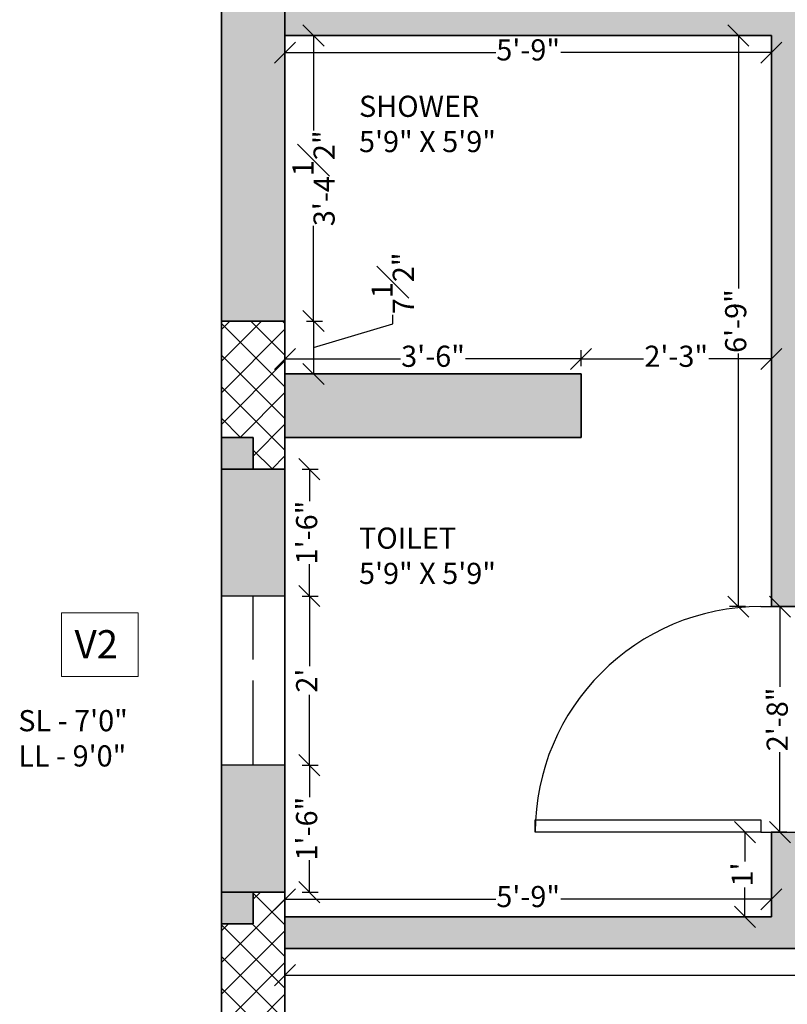
# Model space of a CAD drawing. Units: inches. Extents: x 1365 to 2091, y 1589 to 2091.
# Tile 2 of 8: x 1365 to 1474, y 1792 to 1932. Entities that reach past the tile are written whole.
import ezdxf

# ---------------------------------------------------------------- set-up
doc = ezdxf.new("R2010")
doc.units = ezdxf.units.IN
doc.linetypes.add('ACAD_ISO02W100', pattern=[15, 12, -3])
for name, color, linetype, lineweight in [('A-ANNO-DIMS', 2, 'Continuous', 18), ('A-ANNO-SYMB', 12, 'Continuous', 18), ('A-AREA-IDEN', 7, 'Continuous', 18), ('A-COLS', 7, 'Continuous', 35), ('A-COLS-MARK-PATT', 114, 'Continuous', 13), ('A-COLS-PATT', 1, 'Continuous', 13), ('A-DOOR', 4, 'Continuous', 25), ('A-GLAZ', 150, 'Continuous', 30), ('A-GLAZ-HIDN', 150, 'ACAD_ISO02W100', 30), ('A-WALL', 7, 'Continuous', 35), ('A-WALL-PATT', 253, 'Continuous', 13)]:
    doc.layers.add(name, color=color, linetype=linetype, lineweight=lineweight)
doc.styles.get("Standard").update_dxf_attribs({"font": 'arial.ttf'})
doc.dimstyles.new('ISO-25', dxfattribs={"dimtxt": 3, "dimasz": 3, "dimexe": 1.25, "dimexo": 0.625, "dimtad": 0, "dimlunit": 4, "dimtxsty": 'Standard', "dimblk": 'OBLIQUE', "dimcen": 2.5, "dimclrd": 254, "dimclre": 254, "dimclrt": 1, "dimadec": 0, "dimazin": 0, "dimtfac": 1, "dimtmove": 0, "dimatfit": 3, "dimfxl": 1, "dimfxlon": 1, "dimfrac": 1, "dimarcsym": 0})

# ---------------------------------------------------------------- blocks, each defined once
blk = doc.blocks.new('*U4')
for p, q in [((0, 0), (0, -6)), ((32, 0), (32, -6))]:
    blk.add_line(p, q)
blk.add_lwpolyline([(0, 0), (0, 32), (1.75, 32), (1.75, 0)], close=True)
blk.add_arc((0, 0), 32, 0, 90)
blk = doc.blocks.new('_Oblique')
at = {"color": 0, "linetype": 'ByBlock', "lineweight": -2}
blk.add_line((-0.5, -0.5), (0.5, 0.5), dxfattribs=at)
blk = doc.blocks.new('*D23')
at = {"layer": 'A-ANNO-DIMS', "color": 0, "lineweight": -2, "transparency": 16777216}
for p, q in [((1402.75, 1927.94), (1402.75, 1925.69)), ((1471.75, 1927.94), (1471.75, 1925.69)), ((1402.75, 1926.94), (1432.64, 1926.94)), ((1471.75, 1926.94), (1441.87, 1926.94))]:
    blk.add_line(p, q, dxfattribs=at)
at = {"layer": 'Defpoints', "color": 0, "transparency": 16777216}
for p in [(1402.75, 1929.36), (1471.75, 1929.36), (1471.75, 1926.94)]:
    blk.add_point(p, dxfattribs=at)
at = {"layer": 'A-ANNO-DIMS', "color": 0, "lineweight": -2, "transparency": 16777216, "xscale": 3, "yscale": 3, "zscale": 3, "rotation": 180}
blk.add_blockref('_Oblique', (1402.75, 1926.94), dxfattribs=at)
at = {"layer": 'A-ANNO-DIMS', "color": 0, "lineweight": -2, "transparency": 16777216, "xscale": 3, "yscale": 3, "zscale": 3}
blk.add_blockref('_Oblique', (1471.75, 1926.94), dxfattribs=at)
at = {"layer": 'A-ANNO-DIMS', "color": 0, "transparency": 16777216, "insert": (1437.25, 1926.94), "char_height": 3, "attachment_point": 5}
blk.add_mtext('5\'-9"', dxfattribs=at)
blk = doc.blocks.new('*D24')
at = {"layer": 'A-ANNO-DIMS', "color": 0, "lineweight": -2, "transparency": 16777216}
for p, q in [((1405.8, 1929.36), (1408.05, 1929.36)), ((1406.8, 1929.36), (1406.8, 1915.87)), ((1406.8, 1888.86), (1406.8, 1902.35)), ((1405.8, 1888.86), (1408.05, 1888.86))]:
    blk.add_line(p, q, dxfattribs=at)
at = {"layer": 'Defpoints', "color": 0, "transparency": 16777216}
for p in [(1402.75, 1929.36), (1402.75, 1888.86), (1406.8, 1888.86)]:
    blk.add_point(p, dxfattribs=at)
at = {"layer": 'A-ANNO-DIMS', "color": 0, "lineweight": -2, "transparency": 16777216, "xscale": 3, "yscale": 3, "zscale": 3}
for p, rotation in [((1406.8, 1929.36), 90), ((1406.8, 1888.86), 270)]:
    blk.add_blockref('_Oblique', p, dxfattribs=dict(at, rotation=rotation))
at = {"layer": 'A-ANNO-DIMS', "color": 0, "transparency": 16777216, "insert": (1406.8, 1909.11), "char_height": 3, "attachment_point": 5, "rotation": 90}
blk.add_mtext('3\'-4{\\H1x;\\S1#2;}"', dxfattribs=at)
blk = doc.blocks.new('*D25')
at = {"layer": 'A-ANNO-DIMS', "color": 0, "lineweight": -2, "transparency": 16777216}
for p, q in [((1418.03, 1888.47), (1418.03, 1889.72)), ((1405.8, 1888.86), (1408.05, 1888.86)), ((1406.8, 1888.86), (1406.8, 1881.36)), ((1406.8, 1885.11), (1418.03, 1888.47)), ((1405.8, 1881.36), (1408.05, 1881.36))]:
    blk.add_line(p, q, dxfattribs=at)
at = {"layer": 'Defpoints', "color": 0, "transparency": 16777216}
for p in [(1402.75, 1888.86), (1402.75, 1881.36), (1406.8, 1881.36)]:
    blk.add_point(p, dxfattribs=at)
at = {"layer": 'A-ANNO-DIMS', "color": 0, "lineweight": -2, "transparency": 16777216, "xscale": 3, "yscale": 3, "zscale": 3}
for p, rotation in [((1406.8, 1888.86), 90), ((1406.8, 1881.36), 270)]:
    blk.add_blockref('_Oblique', p, dxfattribs=dict(at, rotation=rotation))
at = {"layer": 'A-ANNO-DIMS', "color": 0, "transparency": 16777216, "insert": (1418.03, 1894.21), "char_height": 3, "attachment_point": 5, "rotation": 90}
blk.add_mtext('7{\\H1x;\\S1#2;}"', dxfattribs=at)
blk = doc.blocks.new('*D26')
at = {"layer": 'A-ANNO-DIMS', "color": 0, "lineweight": -2, "transparency": 16777216}
for p, q in [((1402.75, 1882.48), (1402.75, 1884.73)), ((1444.75, 1882.48), (1444.75, 1884.73)), ((1402.75, 1883.48), (1419.14, 1883.48)), ((1444.75, 1883.48), (1428.37, 1883.48))]:
    blk.add_line(p, q, dxfattribs=at)
at = {"layer": 'Defpoints', "color": 0, "transparency": 16777216}
for p in [(1444.75, 1883.48), (1402.75, 1881.36), (1444.75, 1881.36)]:
    blk.add_point(p, dxfattribs=at)
at = {"layer": 'A-ANNO-DIMS', "color": 0, "lineweight": -2, "transparency": 16777216, "xscale": 3, "yscale": 3, "zscale": 3, "rotation": 180}
blk.add_blockref('_Oblique', (1402.75, 1883.48), dxfattribs=at)
at = {"layer": 'A-ANNO-DIMS', "color": 0, "lineweight": -2, "transparency": 16777216, "xscale": 3, "yscale": 3, "zscale": 3}
blk.add_blockref('_Oblique', (1444.75, 1883.48), dxfattribs=at)
at = {"layer": 'A-ANNO-DIMS', "color": 0, "transparency": 16777216, "insert": (1423.75, 1883.48), "char_height": 3, "attachment_point": 5}
blk.add_mtext('3\'-6"', dxfattribs=at)
blk = doc.blocks.new('*D27')
at = {"layer": 'A-ANNO-DIMS', "color": 0, "lineweight": -2, "transparency": 16777216}
for p, q in [((1444.75, 1882.48), (1444.75, 1884.73)), ((1471.75, 1883.48), (1471.75, 1884.73)), ((1444.75, 1883.48), (1453.62, 1883.48)), ((1471.75, 1883.48), (1462.89, 1883.48))]:
    blk.add_line(p, q, dxfattribs=at)
at = {"layer": 'Defpoints', "color": 0, "transparency": 16777216}
for p in [(1471.75, 1883.48), (1471.75, 1883.48), (1444.75, 1881.36)]:
    blk.add_point(p, dxfattribs=at)
at = {"layer": 'A-ANNO-DIMS', "color": 0, "lineweight": -2, "transparency": 16777216, "xscale": 3, "yscale": 3, "zscale": 3, "rotation": 180}
blk.add_blockref('_Oblique', (1444.75, 1883.48), dxfattribs=at)
at = {"layer": 'A-ANNO-DIMS', "color": 0, "lineweight": -2, "transparency": 16777216, "xscale": 3, "yscale": 3, "zscale": 3}
blk.add_blockref('_Oblique', (1471.75, 1883.48), dxfattribs=at)
at = {"layer": 'A-ANNO-DIMS', "color": 0, "transparency": 16777216, "insert": (1458.25, 1883.48), "char_height": 3, "attachment_point": 5}
blk.add_mtext('2\'-3"', dxfattribs=at)
blk = doc.blocks.new('*D28')
at = {"layer": 'A-ANNO-DIMS', "color": 0, "lineweight": -2, "transparency": 16777216}
for p, q in [((1468.07, 1929.36), (1465.82, 1929.36)), ((1467.07, 1929.36), (1467.07, 1893.48)), ((1467.07, 1848.36), (1467.07, 1884.24)), ((1468.07, 1848.36), (1465.82, 1848.36))]:
    blk.add_line(p, q, dxfattribs=at)
at = {"layer": 'Defpoints', "color": 0, "transparency": 16777216}
for p in [(1471.75, 1929.36), (1467.07, 1848.36), (1471.75, 1848.36)]:
    blk.add_point(p, dxfattribs=at)
at = {"layer": 'A-ANNO-DIMS', "color": 0, "lineweight": -2, "transparency": 16777216, "xscale": 3, "yscale": 3, "zscale": 3}
for p, rotation in [((1467.07, 1929.36), 90), ((1467.07, 1848.36), 270)]:
    blk.add_blockref('_Oblique', p, dxfattribs=dict(at, rotation=rotation))
at = {"layer": 'A-ANNO-DIMS', "color": 0, "transparency": 16777216, "insert": (1467.07, 1888.86), "char_height": 3, "attachment_point": 5, "rotation": 90}
blk.add_mtext('6\'-9"', dxfattribs=at)
blk = doc.blocks.new('*D29')
at = {"layer": 'A-ANNO-DIMS', "color": 0, "lineweight": -2, "transparency": 16777216}
for p, q in [((1405.21, 1867.86), (1407.46, 1867.86)), ((1406.21, 1867.86), (1406.21, 1863.33)), ((1406.21, 1849.86), (1406.21, 1854.39)), ((1405.21, 1849.86), (1407.46, 1849.86))]:
    blk.add_line(p, q, dxfattribs=at)
at = {"layer": 'Defpoints', "color": 0, "transparency": 16777216}
for p in [(1402.75, 1867.86), (1402.75, 1849.86), (1406.21, 1849.86)]:
    blk.add_point(p, dxfattribs=at)
at = {"layer": 'A-ANNO-DIMS', "color": 0, "lineweight": -2, "transparency": 16777216, "xscale": 3, "yscale": 3, "zscale": 3}
for p, rotation in [((1406.21, 1867.86), 90), ((1406.21, 1849.86), 270)]:
    blk.add_blockref('_Oblique', p, dxfattribs=dict(at, rotation=rotation))
at = {"layer": 'A-ANNO-DIMS', "color": 0, "transparency": 16777216, "insert": (1406.21, 1858.86), "char_height": 3, "attachment_point": 5, "rotation": 90}
blk.add_mtext('1\'-6"', dxfattribs=at)
blk = doc.blocks.new('*D30')
at = {"layer": 'A-ANNO-DIMS', "color": 0, "lineweight": -2, "transparency": 16777216}
for p, q in [((1405.21, 1849.86), (1407.46, 1849.86)), ((1406.21, 1849.86), (1406.21, 1839.89)), ((1406.21, 1825.86), (1406.21, 1835.83)), ((1405.21, 1825.86), (1407.46, 1825.86))]:
    blk.add_line(p, q, dxfattribs=at)
at = {"layer": 'Defpoints', "color": 0, "transparency": 16777216}
for p in [(1402.75, 1849.86), (1402.75, 1825.86), (1406.21, 1825.86)]:
    blk.add_point(p, dxfattribs=at)
at = {"layer": 'A-ANNO-DIMS', "color": 0, "lineweight": -2, "transparency": 16777216, "xscale": 3, "yscale": 3, "zscale": 3}
for p, rotation in [((1406.21, 1849.86), 90), ((1406.21, 1825.86), 270)]:
    blk.add_blockref('_Oblique', p, dxfattribs=dict(at, rotation=rotation))
at = {"layer": 'A-ANNO-DIMS', "color": 0, "transparency": 16777216, "insert": (1406.21, 1837.86), "char_height": 3, "attachment_point": 5, "rotation": 90}
blk.add_mtext("2'", dxfattribs=at)
blk = doc.blocks.new('*D31')
at = {"layer": 'A-ANNO-DIMS', "color": 0, "lineweight": -2, "transparency": 16777216}
for p, q in [((1405.21, 1825.86), (1407.46, 1825.86)), ((1406.21, 1825.86), (1406.21, 1821.33)), ((1406.21, 1807.86), (1406.21, 1812.39)), ((1405.21, 1807.86), (1407.46, 1807.86))]:
    blk.add_line(p, q, dxfattribs=at)
at = {"layer": 'Defpoints', "color": 0, "transparency": 16777216}
for p in [(1402.75, 1825.86), (1402.75, 1807.86), (1406.21, 1807.86)]:
    blk.add_point(p, dxfattribs=at)
at = {"layer": 'A-ANNO-DIMS', "color": 0, "lineweight": -2, "transparency": 16777216, "xscale": 3, "yscale": 3, "zscale": 3}
for p, rotation in [((1406.21, 1825.86), 90), ((1406.21, 1807.86), 270)]:
    blk.add_blockref('_Oblique', p, dxfattribs=dict(at, rotation=rotation))
at = {"layer": 'A-ANNO-DIMS', "color": 0, "transparency": 16777216, "insert": (1406.21, 1816.86), "char_height": 3, "attachment_point": 5, "rotation": 90}
blk.add_mtext('1\'-6"', dxfattribs=at)
blk = doc.blocks.new('*D32')
at = {"layer": 'A-ANNO-DIMS', "color": 0, "lineweight": -2, "transparency": 16777216}
for p, q in [((1402.75, 1805.84), (1402.75, 1808.09)), ((1471.75, 1805.84), (1471.75, 1808.09)), ((1402.75, 1806.84), (1432.64, 1806.84)), ((1471.75, 1806.84), (1441.87, 1806.84))]:
    blk.add_line(p, q, dxfattribs=at)
at = {"layer": 'Defpoints', "color": 0, "transparency": 16777216}
for p in [(1471.75, 1806.84), (1402.75, 1804.36), (1471.75, 1804.36)]:
    blk.add_point(p, dxfattribs=at)
at = {"layer": 'A-ANNO-DIMS', "color": 0, "lineweight": -2, "transparency": 16777216, "xscale": 3, "yscale": 3, "zscale": 3, "rotation": 180}
blk.add_blockref('_Oblique', (1402.75, 1806.84), dxfattribs=at)
at = {"layer": 'A-ANNO-DIMS', "color": 0, "lineweight": -2, "transparency": 16777216, "xscale": 3, "yscale": 3, "zscale": 3}
blk.add_blockref('_Oblique', (1471.75, 1806.84), dxfattribs=at)
at = {"layer": 'A-ANNO-DIMS', "color": 0, "transparency": 16777216, "insert": (1437.25, 1806.84), "char_height": 3, "attachment_point": 5}
blk.add_mtext('5\'-9"', dxfattribs=at)
blk = doc.blocks.new('*D33')
at = {"layer": 'A-ANNO-DIMS', "color": 0, "lineweight": -2, "transparency": 16777216}
for p, q in [((1468.99, 1816.36), (1466.74, 1816.36)), ((1467.99, 1816.36), (1467.99, 1812.22)), ((1467.99, 1804.36), (1467.99, 1808.49)), ((1468.99, 1804.36), (1466.74, 1804.36))]:
    blk.add_line(p, q, dxfattribs=at)
at = {"layer": 'Defpoints', "color": 0, "transparency": 16777216}
for p in [(1471.75, 1816.36), (1467.99, 1804.36), (1471.75, 1804.36)]:
    blk.add_point(p, dxfattribs=at)
at = {"layer": 'A-ANNO-DIMS', "color": 0, "lineweight": -2, "transparency": 16777216, "xscale": 3, "yscale": 3, "zscale": 3}
for p, rotation in [((1467.99, 1816.36), 90), ((1467.99, 1804.36), 270)]:
    blk.add_blockref('_Oblique', p, dxfattribs=dict(at, rotation=rotation))
at = {"layer": 'A-ANNO-DIMS', "color": 0, "transparency": 16777216, "insert": (1467.99, 1810.36), "char_height": 3, "attachment_point": 5, "rotation": 90}
blk.add_mtext("1'", dxfattribs=at)
blk = doc.blocks.new('*D34')
at = {"layer": 'A-ANNO-DIMS', "color": 0, "lineweight": -2, "transparency": 16777216}
for p, q in [((1473.96, 1848.36), (1471.71, 1848.36)), ((1472.96, 1848.36), (1472.96, 1837)), ((1472.96, 1816.36), (1472.96, 1827.72)), ((1473.96, 1816.36), (1471.71, 1816.36))]:
    blk.add_line(p, q, dxfattribs=at)
at = {"layer": 'Defpoints', "color": 0, "transparency": 16777216}
for p in [(1472.96, 1848.36), (1476.25, 1848.36), (1476.25, 1816.36)]:
    blk.add_point(p, dxfattribs=at)
at = {"layer": 'A-ANNO-DIMS', "color": 0, "lineweight": -2, "transparency": 16777216, "xscale": 3, "yscale": 3, "zscale": 3}
for p, rotation in [((1472.96, 1848.36), 90), ((1472.96, 1816.36), 270)]:
    blk.add_blockref('_Oblique', p, dxfattribs=dict(at, rotation=rotation))
at = {"layer": 'A-ANNO-DIMS', "color": 0, "transparency": 16777216, "insert": (1472.96, 1832.36), "char_height": 3, "attachment_point": 5, "rotation": 90}
blk.add_mtext('2\'-8"', dxfattribs=at)
blk = doc.blocks.new('*D40')
at = {"layer": 'A-ANNO-DIMS', "color": 0, "lineweight": -2, "transparency": 16777216}
for p, q in [((1402.75, 1797.07), (1402.75, 1794.82)), ((1402.75, 1796.07), (1512.62, 1796.07)), ((1633.75, 1796.07), (1523.89, 1796.07)), ((1633.75, 1797.07), (1633.75, 1794.82))]:
    blk.add_line(p, q, dxfattribs=at)
at = {"layer": 'Defpoints', "color": 0, "transparency": 16777216}
for p in [(1402.75, 1799.86), (1633.75, 1798.86), (1633.75, 1796.07)]:
    blk.add_point(p, dxfattribs=at)
at = {"layer": 'A-ANNO-DIMS', "color": 0, "lineweight": -2, "transparency": 16777216, "xscale": 3, "yscale": 3, "zscale": 3, "rotation": 180}
blk.add_blockref('_Oblique', (1402.75, 1796.07), dxfattribs=at)
at = {"layer": 'A-ANNO-DIMS', "color": 0, "lineweight": -2, "transparency": 16777216, "xscale": 3, "yscale": 3, "zscale": 3}
blk.add_blockref('_Oblique', (1633.75, 1796.07), dxfattribs=at)
at = {"layer": 'A-ANNO-DIMS', "color": 0, "transparency": 16777216, "insert": (1518.25, 1796.07), "char_height": 3, "attachment_point": 5}
blk.add_mtext('19\'-3"', dxfattribs=at)
blk = doc.blocks.new('OPENING-TAG-V2')
blk.add_lwpolyline([(6.13, 13.79), (17.02, 13.79), (17.02, 4.75), (6.13, 4.75)], close=True)
at = {"attachment_point": 1}
for s, width, insert, char_height in [('{V2}', 14.5136, (7.98, 11.34), 4), ('{SL - 7\'0"\\PLL - 9\'0"}', 24.3857, (0, 0), 3)]:
    blk.add_mtext_dynamic_manual_height_columns(s, width=width, gutter_width=12.5, heights=[0], dxfattribs=dict(at, insert=insert, char_height=char_height))

msp = doc.modelspace()

# ---------------------------------------------------------------- hatches: boundary and pattern name
at = {"layer": 'A-COLS-MARK-PATT'}
h = msp.add_hatch(color=256, dxfattribs=at)
h.dxf.hatch_style = 1
h.paths.add_polyline_path([(1398.254, 2062.858), (1393.754, 2062.858), (1393.754, 2058.358), (1398.254, 2058.358)])
h.paths.add_polyline_path([(1398.254, 1872.358), (1393.754, 1872.358), (1393.754, 1867.858), (1398.254, 1867.858)])
h.paths.add_polyline_path([(1398.254, 1807.858), (1393.754, 1807.858), (1393.754, 1803.358), (1398.254, 1803.358)])
h.paths.add_polyline_path([(1398.254, 1647.358), (1393.754, 1647.358), (1393.754, 1642.858), (1398.254, 1642.858)])
h.paths.add_polyline_path([(1638.254, 1647.358), (1633.754, 1647.358), (1633.754, 1642.858), (1638.254, 1642.858)])
h.paths.add_polyline_path([(1638.254, 1732.858), (1633.754, 1732.858), (1633.754, 1728.358), (1638.254, 1728.358)])
h.paths.add_polyline_path([(1647.254, 1876.858), (1642.754, 1876.858), (1642.754, 1872.358), (1647.254, 1872.358)])
h.paths.add_polyline_path([(1647.254, 1803.358), (1642.754, 1803.358), (1642.754, 1798.858), (1647.254, 1798.858)])
h.paths.add_polyline_path([(1647.254, 2062.858), (1642.754, 2062.858), (1642.754, 2058.358), (1647.254, 2058.358)])
h.paths.add_polyline_path([(1824.254, 2062.858), (1819.754, 2062.858), (1819.754, 2058.358), (1824.254, 2058.358)])
h.paths.add_polyline_path([(1824.254, 1885.858), (1819.754, 1885.858), (1819.754, 1881.358), (1824.254, 1881.358)])
h.paths.add_polyline_path([(1828.754, 1647.358), (1824.254, 1647.358), (1824.254, 1642.858), (1828.754, 1642.858)])
h.paths.add_polyline_path([(1948.754, 1647.358), (1944.254, 1647.358), (1944.254, 1642.858), (1948.754, 1642.858)])
h.paths.add_polyline_path([(2041.754, 1647.358), (2037.254, 1647.358), (2037.254, 1642.858), (2041.754, 1642.858)])
h.paths.add_polyline_path([(2041.754, 1885.858), (2037.254, 1885.858), (2037.254, 1881.358), (2041.754, 1881.358)])
h.paths.add_polyline_path([(2041.754, 2062.858), (2037.254, 2062.858), (2037.254, 2058.358), (2041.754, 2058.358)])
at = {"layer": 'A-COLS-PATT'}
h = msp.add_hatch(dxfattribs=at)
h.set_pattern_fill('ANSI37', color=256)
h.paths.add_polyline_path([(1414.754, 2062.858), (1398.254, 2062.858), (1398.254, 2058.358), (1393.754, 2058.358), (1393.754, 2053.858), (1414.754, 2053.858)])
h.paths.add_polyline_path([(1402.754, 1888.858), (1393.754, 1888.858), (1393.754, 1872.358), (1398.254, 1872.358), (1398.254, 1867.858), (1402.754, 1867.858), (1402.754, 1872.358)])
h.paths.add_polyline_path([(1402.754, 1807.858), (1398.254, 1807.858), (1398.254, 1803.358), (1393.754, 1803.358), (1393.754, 1789.858), (1402.754, 1789.858)])
h.paths.add_polyline_path([(1402.754, 1663.858), (1393.754, 1663.858), (1393.754, 1647.358), (1398.254, 1647.358), (1398.254, 1642.858), (1402.754, 1642.858)])
h.paths.add_polyline_path([(1638.254, 1666.858), (1629.254, 1666.858), (1629.254, 1642.858), (1633.754, 1642.858), (1633.754, 1647.358), (1638.254, 1647.358)])
h.paths.add_polyline_path([(1633.754, 1732.858), (1629.254, 1732.858), (1629.254, 1714.858), (1633.754, 1714.858)])
h.paths.add_polyline_path([(1638.254, 1728.358), (1633.754, 1728.358), (1633.754, 1714.858), (1638.254, 1714.858)])
at = {"layer": 'A-WALL-PATT'}
h = msp.add_hatch(color=256, dxfattribs=at)
h.dxf.hatch_style = 1
h.paths.add_polyline_path([(1402.754, 2053.858), (1393.754, 2053.858), (1393.754, 2029.858), (1402.754, 2029.858)])
h.paths.add_polyline_path([(1402.754, 2005.858), (1393.754, 2005.858), (1393.754, 1888.858), (1402.754, 1888.858)])
h.paths.add_polyline_path([(1444.754, 1984.858), (1402.754, 1984.858), (1402.754, 1975.858), (1444.754, 1975.858)], flags=17)
h.paths.add_polyline_path([(1476.254, 1993.858), (1471.754, 1993.858), (1471.754, 1933.858), (1402.754, 1933.858), (1402.754, 1929.358), (1471.754, 1929.358), (1471.754, 1848.358), (1476.254, 1848.358), (1476.254, 1872.358), (1569.254, 1872.358), (1569.254, 1798.858), (1573.754, 1798.858), (1629.254, 1798.858), (1629.254, 1807.858), (1578.254, 1807.858), (1578.254, 1867.858), (1623.254, 1867.858), (1623.254, 1876.858), (1476.254, 1876.858)])
h.paths.add_polyline_path([(1402.754, 1867.858), (1393.754, 1867.858), (1393.754, 1849.858), (1402.754, 1849.858)])
h.paths.add_polyline_path([(1402.754, 1825.858), (1393.754, 1825.858), (1393.754, 1807.858), (1398.254, 1807.858), (1402.754, 1807.858)])
h = msp.add_hatch(color=256, dxfattribs=at)
h.dxf.hatch_style = 1
h.paths.add_polyline_path([(1444.754, 1881.358), (1402.754, 1881.358), (1402.754, 1872.358), (1444.754, 1872.358)])
h = msp.add_hatch(color=256, dxfattribs=at)
h.dxf.hatch_style = 1
h.paths.add_polyline_path([(1402.754, 1753.858), (1393.754, 1753.858), (1393.754, 1663.858), (1402.754, 1663.858)])
h.paths.add_polyline_path([(1533.254, 1804.358), (1476.254, 1804.358), (1476.254, 1816.358), (1471.754, 1816.358), (1471.754, 1804.358), (1402.754, 1804.358), (1402.754, 1799.858), (1533.254, 1799.858)])
h.paths.add_polyline_path([(1638.254, 1714.858), (1633.754, 1714.858), (1633.754, 1666.858), (1638.254, 1666.858)])
h.paths.add_polyline_path([(1638.254, 1740.858), (1633.754, 1740.858), (1633.754, 1732.858), (1638.254, 1732.858)])
h.paths.add_polyline_path([(1954.754, 1744.858), (1948.754, 1744.858), (1944.254, 1744.858), (1824.254, 1744.858), (1824.254, 1821.858), (1819.754, 1821.858), (1819.754, 1666.858), (1824.254, 1666.858), (1824.254, 1740.358), (1944.254, 1740.358), (1948.754, 1740.358), (1954.754, 1740.358)])
h.paths.add_polyline_path([(1948.754, 1698.358), (1944.254, 1698.358), (1944.254, 1651.858), (1948.754, 1651.858)])
h.paths.add_polyline_path([(1948.754, 1740.358), (1944.254, 1740.358), (1944.254, 1734.358), (1948.754, 1734.358)], flags=17)

# ---------------------------------------------------------------- linework, layer by layer
at = {"layer": 'A-COLS'}
for p, q in [((1393.754, 1888.858), (1402.754, 1888.858)), ((1393.754, 1867.858), (1393.754, 1872.358)), ((1393.754, 1872.358), (1398.254, 1872.358)), ((1398.254, 1872.358), (1398.254, 1867.858)), ((1402.754, 1872.358), (1402.754, 1867.858)), ((1402.754, 1867.858), (1393.754, 1867.858)), ((1402.754, 1807.858), (1393.754, 1807.858)), ((1393.754, 1807.858), (1398.254, 1807.858)), ((1398.254, 1807.858), (1398.254, 1803.358)), ((1398.254, 1803.358), (1393.754, 1803.358))]:
    msp.add_line(p, q, dxfattribs=at)
at = {"layer": 'A-GLAZ'}
for p, q in [((1402.754, 1849.858), (1393.754, 1849.858)), ((1402.754, 1825.858), (1393.754, 1825.858))]:
    msp.add_line(p, q, dxfattribs=at)
at = {"layer": 'A-GLAZ-HIDN'}
msp.add_line((1398.254, 1825.858), (1398.254, 1849.858), dxfattribs=at)
at = {"layer": 'A-WALL'}
for p, q in [((1393.754, 1642.858), (1393.754, 2062.858)), ((1402.754, 1807.858), (1402.754, 2053.858)), ((1402.754, 1929.358), (1471.754, 1929.358)), ((1471.754, 1929.358), (1471.754, 1848.358)), ((1402.754, 1881.358), (1444.754, 1881.358)), ((1444.754, 1881.358), (1444.754, 1872.358)), ((1444.754, 1872.358), (1402.754, 1872.358)), ((1471.754, 1848.358), (1476.254, 1848.358)), ((1471.754, 1804.358), (1471.754, 1816.358)), ((1402.754, 1642.858), (1402.754, 1807.858)), ((1402.754, 1804.358), (1471.754, 1804.358)), ((1533.254, 1799.858), (1402.754, 1799.858))]:
    msp.add_line(p, q, dxfattribs=at)

# ---------------------------------------------------------------- block references
at = {"layer": 'A-ANNO-SYMB'}
msp.add_blockref('OPENING-TAG-V2', (1364.926, 1833.676), dxfattribs=at)
at = {"layer": 'A-DOOR', "rotation": 89.99999999999999}
msp.add_blockref('*U4', (1470.254, 1816.358), dxfattribs=at)

# ---------------------------------------------------------------- texts
at = {"layer": 'A-AREA-IDEN', "char_height": 3, "attachment_point": 1}
for s, insert in [('{SHOWER\\P5\'9" X 5\'9"}', (1413.254, 1920.822)), ('{TOILET\\P5\'9" X 5\'9"}', (1413.254, 1859.567))]:
    msp.add_mtext_dynamic_manual_height_columns(s, width=33.58604, gutter_width=12.5, heights=[0], dxfattribs=dict(at, insert=insert))

# ---------------------------------------------------------------- dimensions: what is measured, and where the dimension line sits
at = {"layer": 'A-ANNO-DIMS'}
for base, p1, p2, override, picture, middle in [((1406.801, 1888.858), (1402.754, 1929.358), (1402.754, 1888.858), {"dimclrd": 0, "dimclre": 0, "dimclrt": 0}, '*D24', (1406.801, 1909.108)), ((1467.073, 1848.358), (1471.754, 1929.358), (1471.754, 1848.358), {"dimclrd": 0, "dimclre": 0, "dimclrt": 0}, '*D28', (1467.073, 1888.858)), ((1406.801, 1881.358), (1402.754, 1888.858), (1402.754, 1881.358), {"dimclrd": 0, "dimclre": 0, "dimclrt": 0, "dimtmove": 1}, '*D25', (1418.025, 1890.35)), ((1406.208, 1849.858), (1402.754, 1867.858), (1402.754, 1849.858), {"dimclrd": 0, "dimclre": 0, "dimclrt": 0}, '*D29', (1406.208, 1858.858)), ((1406.208, 1825.858), (1402.754, 1849.858), (1402.754, 1825.858), {"dimclrd": 0, "dimclre": 0, "dimclrt": 0, "dimtmove": 1}, '*D30', (1406.208, 1837.858)), ((1472.962, 1848.358), (1476.254, 1816.358), (1476.254, 1848.358), {"dimclrd": 0, "dimclre": 0, "dimclrt": 0}, '*D34', (1472.962, 1832.358)), ((1406.208, 1807.858), (1402.754, 1825.858), (1402.754, 1807.858), {"dimclrd": 0, "dimclre": 0, "dimclrt": 0, "dimtmove": 1}, '*D31', (1406.208, 1816.858)), ((1467.989, 1804.358), (1471.754, 1816.358), (1471.754, 1804.358), {"dimclrd": 0, "dimclre": 0, "dimclrt": 0}, '*D33', (1467.989, 1810.358))]:
    dim = msp.add_linear_dim(base=base, p1=p1, p2=p2, angle=90, dimstyle='ISO-25', override=override, dxfattribs=at)
    dim.commit()
    dim.dimension.update_dxf_attribs({"geometry": picture, "text_midpoint": middle})
for base, p1, p2, override, picture, middle in [((1471.754, 1926.944), (1402.754, 1929.358), (1471.754, 1929.358), {"dimclrd": 0, "dimclre": 0, "dimclrt": 0}, '*D23', (1437.254, 1926.944)), ((1444.754, 1883.475), (1402.754, 1881.358), (1444.754, 1881.358), {"dimclrd": 0, "dimclre": 0, "dimclrt": 0}, '*D26', (1423.754, 1883.475)), ((1471.754, 1883.475), (1444.754, 1881.358), (1471.754, 1883.475), {"dimclrd": 0, "dimclre": 0, "dimclrt": 0, "dimtmove": 1}, '*D27', (1458.254, 1883.475)), ((1471.754, 1806.844), (1402.754, 1804.358), (1471.754, 1804.358), {"dimclrd": 0, "dimclre": 0, "dimclrt": 0}, '*D32', (1437.254, 1806.844)), ((1633.754, 1796.07), (1402.754, 1799.858), (1633.754, 1798.858), {"dimclrd": 0, "dimclre": 0, "dimclrt": 0}, '*D40', (1518.254, 1796.07))]:
    dim = msp.add_linear_dim(base=base, p1=p1, p2=p2, dimstyle='ISO-25', override=override, dxfattribs=at)
    dim.commit()
    dim.dimension.update_dxf_attribs({"geometry": picture, "text_midpoint": middle})

doc.saveas('drawing.dxf')
